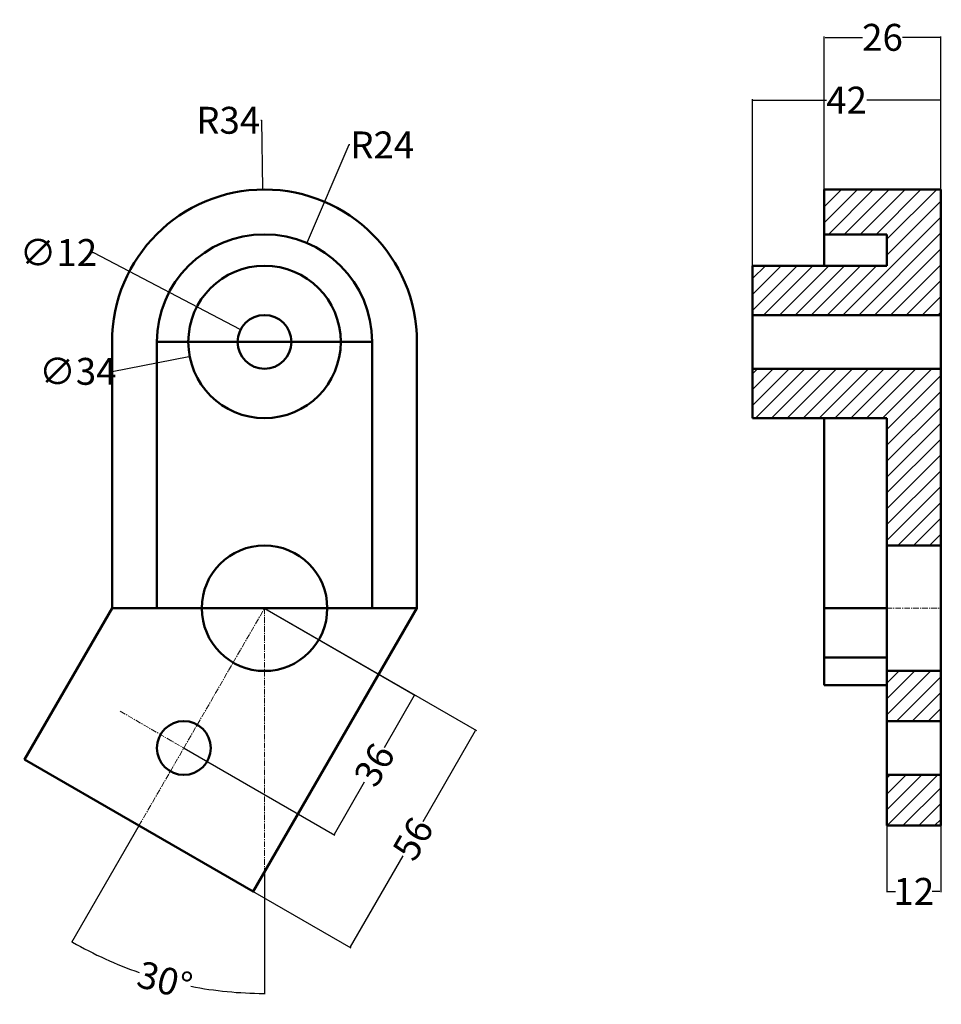
# Model space of a CAD drawing. Units: millimetres. Extents: x 37 to 242, y 56 to 275.
import ezdxf

# ---------------------------------------------------------------- set-up
doc = ezdxf.new("R2010")
doc.units = ezdxf.units.MM
doc.header["$MEASUREMENT"] = 0
doc.linetypes.add('CENTER', pattern=[2, 1.25, -0.25, 0.25, -0.25])
for name, color, linetype, lineweight in [('M-CNTR', 1, 'CENTER', 18), ('M-DIMS', 2, 'Continuous', 25), ('M-HATC', 8, 'Continuous', 18), ('M-OUTL', 7, 'Continuous', 50)]:
    doc.layers.add(name, color=color, linetype=linetype, lineweight=lineweight)
doc.styles.get("Standard").update_dxf_attribs({"font": 'arial.ttf'})
doc.dimstyles.get("Standard").update_dxf_attribs({"dimtxt": 6, "dimasz": 0.18, "dimexe": 0.18, "dimexo": 0.0625, "dimgap": 0.09, "dimtad": 0, "dimtoh": 1, "dimdec": 0, "dimzin": 0, "dimdsep": 46, "dimtxsty": 'Standard', "dimcen": 0.09, "dimadec": 0, "dimazin": 0, "dimtfac": 1, "dimtdec": 0, "dimtofl": 0, "dimtmove": 0, "dimatfit": 3, "dimfxl": 1, "dimtolj": 1, "dimtzin": 0, "dimarcsym": 0})

# ---------------------------------------------------------------- blocks, each defined once
blk = doc.blocks.new('*D1')
at = {"layer": 'Defpoints', "color": 0, "transparency": 16777216}
for p in [(90.71, 237.56), (91.17, 203.56)]:
    blk.add_point(p, dxfattribs=at)
at = {"layer": 'M-DIMS', "color": 0, "lineweight": -2, "transparency": 16777216}
for p, q in [((90.32, 253), (90.5, 253)), ((90.5, 253), (90.71, 237.74)), ((91.08, 203.56), (91.26, 203.56)), ((91.17, 203.47), (91.17, 203.65))]:
    blk.add_line(p, q, dxfattribs=at)
at = {"layer": 'M-DIMS', "color": 0, "transparency": 16777216}
blk.add_solid([(90.74, 237.74), (90.68, 237.74), (90.71, 237.56)], dxfattribs=at)
at = {"layer": 'M-DIMS', "color": 0, "transparency": 16777216, "insert": (83.07, 253), "char_height": 6, "attachment_point": 5}
blk.add_mtext('\\A1;R34', dxfattribs=at)
blk = doc.blocks.new('*D2')
at = {"layer": 'Defpoints', "color": 0, "transparency": 16777216}
for p in [(100.62, 225.62), (91.17, 203.56)]:
    blk.add_point(p, dxfattribs=at)
at = {"layer": 'M-DIMS', "color": 0, "lineweight": -2, "transparency": 16777216}
for p, q in [((110, 247.5), (100.69, 225.79)), ((110.18, 247.5), (110, 247.5)), ((91.08, 203.56), (91.26, 203.56)), ((91.17, 203.47), (91.17, 203.65))]:
    blk.add_line(p, q, dxfattribs=at)
at = {"layer": 'M-DIMS', "color": 0, "transparency": 16777216}
blk.add_solid([(100.67, 225.8), (100.72, 225.77), (100.62, 225.62)], dxfattribs=at)
at = {"layer": 'M-DIMS', "color": 0, "transparency": 16777216, "insert": (117.43, 247.5), "char_height": 6, "attachment_point": 5}
blk.add_mtext('\\A1;R24', dxfattribs=at)
blk = doc.blocks.new('*D3')
at = {"layer": 'Defpoints', "color": 0, "transparency": 16777216}
for p in [(242, 257.5), (200, 220.56), (242, 220.56)]:
    blk.add_point(p, dxfattribs=at)
at = {"layer": 'M-DIMS', "color": 0, "lineweight": -2, "transparency": 16777216}
for p, q in [((200, 220.62), (200, 257.68)), ((200.18, 257.5), (216.52, 257.5)), ((241.82, 257.5), (225.48, 257.5)), ((242, 220.62), (242, 257.68))]:
    blk.add_line(p, q, dxfattribs=at)
at = {"layer": 'M-DIMS', "color": 0, "transparency": 16777216}
for points in [[(200.18, 257.53), (200.18, 257.47), (200, 257.5)], [(241.82, 257.53), (241.82, 257.47), (242, 257.5)]]:
    blk.add_solid(points, dxfattribs=at)
at = {"layer": 'M-DIMS', "color": 0, "transparency": 16777216, "insert": (221, 257.5), "char_height": 6, "attachment_point": 5}
blk.add_mtext('\\A1;42', dxfattribs=at)
blk = doc.blocks.new('*D4')
at = {"layer": 'Defpoints', "color": 0, "transparency": 16777216}
for p in [(242, 271.5), (216, 237.56), (242, 237.56)]:
    blk.add_point(p, dxfattribs=at)
at = {"layer": 'M-DIMS', "color": 0, "lineweight": -2, "transparency": 16777216}
for p, q in [((216, 237.62), (216, 271.68)), ((216.18, 271.5), (224.56, 271.5)), ((241.82, 271.5), (233.44, 271.5)), ((242, 237.62), (242, 271.68))]:
    blk.add_line(p, q, dxfattribs=at)
at = {"layer": 'M-DIMS', "color": 0, "transparency": 16777216}
for points in [[(216.18, 271.53), (216.18, 271.47), (216, 271.5)], [(241.82, 271.53), (241.82, 271.47), (242, 271.5)]]:
    blk.add_solid(points, dxfattribs=at)
at = {"layer": 'M-DIMS', "color": 0, "transparency": 16777216, "insert": (229, 271.5), "char_height": 6, "attachment_point": 5}
blk.add_mtext('\\A1;26', dxfattribs=at)
blk = doc.blocks.new('*D5')
at = {"layer": 'Defpoints', "color": 0, "transparency": 16777216}
for p in [(230, 95.66), (242, 95.66), (242, 81)]:
    blk.add_point(p, dxfattribs=at)
at = {"layer": 'M-DIMS', "color": 0, "lineweight": -2, "transparency": 16777216}
for p, q in [((230, 95.6), (230, 80.82)), ((242, 95.6), (242, 80.82)), ((230.18, 81), (231.93, 81)), ((241.82, 81), (240.07, 81))]:
    blk.add_line(p, q, dxfattribs=at)
at = {"layer": 'M-DIMS', "color": 0, "transparency": 16777216}
for points in [[(230.18, 81.03), (230.18, 80.97), (230, 81)], [(241.82, 81.03), (241.82, 80.97), (242, 81)]]:
    blk.add_solid(points, dxfattribs=at)
at = {"layer": 'M-DIMS', "color": 0, "transparency": 16777216, "insert": (236, 81), "char_height": 6, "attachment_point": 5}
blk.add_mtext('\\A1;12', dxfattribs=at)
blk = doc.blocks.new('*D6')
at = {"layer": 'Defpoints', "color": 0, "transparency": 16777216}
for p in [(107.86, 206.78), (74.47, 200.34)]:
    blk.add_point(p, dxfattribs=at)
at = {"layer": 'M-DIMS', "color": 0, "lineweight": -2, "transparency": 16777216}
for p, q in [((91.08, 203.56), (91.26, 203.56)), ((91.17, 203.47), (91.17, 203.65)), ((57.17, 197), (74.3, 200.31))]:
    blk.add_line(p, q, dxfattribs=at)
at = {"layer": 'M-DIMS', "color": 0, "transparency": 16777216}
blk.add_solid([(74.29, 200.34), (74.3, 200.28), (74.47, 200.34)], dxfattribs=at)
at = {"layer": 'M-DIMS', "color": 0, "transparency": 16777216, "insert": (49.53, 197), "char_height": 6, "attachment_point": 5}
blk.add_mtext('\\A1;∅34', dxfattribs=at)
blk = doc.blocks.new('*D7')
at = {"layer": 'Defpoints', "color": 0, "transparency": 16777216}
for p in [(85.85, 206.34), (96.48, 200.78)]:
    blk.add_point(p, dxfattribs=at)
at = {"layer": 'M-DIMS', "color": 0, "lineweight": -2, "transparency": 16777216}
for p, q in [((52.82, 223.5), (53, 223.5)), ((53, 223.5), (85.69, 206.42)), ((91.08, 203.56), (91.26, 203.56)), ((91.17, 203.47), (91.17, 203.65))]:
    blk.add_line(p, q, dxfattribs=at)
at = {"layer": 'M-DIMS', "color": 0, "transparency": 16777216}
blk.add_solid([(85.7, 206.45), (85.68, 206.4), (85.85, 206.34)], dxfattribs=at)
at = {"layer": 'M-DIMS', "color": 0, "transparency": 16777216, "insert": (45.2, 223.5), "char_height": 6, "attachment_point": 5}
blk.add_mtext('\\A1;∅12', dxfattribs=at)
blk = doc.blocks.new('*D8')
at = {"layer": 'Defpoints', "color": 0, "transparency": 16777216}
for p in [(91.17, 144.16), (63.17, 95.66), (110.27, 68.47)]:
    blk.add_point(p, dxfattribs=at)
at = {"layer": 'M-DIMS', "color": 0, "lineweight": -2, "transparency": 16777216}
for p, q in [((91.22, 144.13), (138.42, 116.88)), ((138.18, 116.81), (126.46, 96.52)), ((63.22, 95.63), (110.42, 68.38)), ((110.36, 68.63), (122.07, 88.92))]:
    blk.add_line(p, q, dxfattribs=at)
at = {"layer": 'M-DIMS', "color": 0, "transparency": 16777216}
for points in [[(138.15, 116.83), (138.2, 116.8), (138.27, 116.97)], [(110.33, 68.64), (110.38, 68.61), (110.27, 68.47)]]:
    blk.add_solid(points, dxfattribs=at)
at = {"layer": 'M-DIMS', "color": 0, "transparency": 16777216, "insert": (124.27, 92.72), "char_height": 6, "attachment_point": 5, "rotation": 60}
blk.add_mtext('\\A1;56', dxfattribs=at)
blk = doc.blocks.new('*D9')
at = {"layer": 'Defpoints', "color": 0, "transparency": 16777216}
for p in [(91.17, 144.16), (73.17, 112.98), (106.66, 93.65)]:
    blk.add_point(p, dxfattribs=at)
at = {"layer": 'M-DIMS', "color": 0, "lineweight": -2, "transparency": 16777216}
for p, q in [((91.22, 144.13), (124.82, 124.73)), ((124.57, 124.67), (117.85, 113.03)), ((73.22, 112.95), (106.82, 93.56)), ((106.75, 93.8), (113.47, 105.44))]:
    blk.add_line(p, q, dxfattribs=at)
at = {"layer": 'M-DIMS', "color": 0, "transparency": 16777216}
for points in [[(124.55, 124.68), (124.6, 124.65), (124.66, 124.82)], [(106.73, 93.82), (106.78, 93.79), (106.66, 93.65)]]:
    blk.add_solid(points, dxfattribs=at)
at = {"layer": 'M-DIMS', "color": 0, "transparency": 16777216, "insert": (115.66, 109.23), "char_height": 6, "attachment_point": 5, "rotation": 60}
blk.add_mtext('\\A1;36', dxfattribs=at)
blk = doc.blocks.new('*D10')
at = {"layer": 'Defpoints', "color": 0, "transparency": 16777216}
for p in [(91.17, 144.16), (91.17, 144.16), (63.17, 95.66), (91.17, 85.27), (61.79, 63.44)]:
    blk.add_point(p, dxfattribs=at)
at = {"layer": 'M-DIMS', "color": 0, "lineweight": -2, "transparency": 16777216}
for p, q in [((63.14, 95.61), (48.12, 69.61)), ((91.17, 85.21), (91.17, 58.08))]:
    blk.add_line(p, q, dxfattribs=at)
for start, end in [(240.1201, 251.0128), (258.9872, 269.8799)]:
    blk.add_arc((91.17, 144.16), 85.91, start, end, dxfattribs=at)
at = {"layer": 'M-DIMS', "color": 0, "transparency": 16777216}
for points in [[(48.36, 69.65), (48.39, 69.7), (48.21, 69.77)], [(90.99, 58.29), (90.99, 58.23), (91.17, 58.26)]]:
    blk.add_solid(points, dxfattribs=at)
at = {"layer": 'M-DIMS', "color": 0, "transparency": 16777216, "insert": (68.93, 61.18), "char_height": 6, "attachment_point": 5, "rotation": 345}
blk.add_mtext('\\A1;30°', dxfattribs=at)

msp = doc.modelspace()

# ---------------------------------------------------------------- hatches: boundary and pattern name
at = {"layer": 'M-HATC'}
h = msp.add_hatch(dxfattribs=at)
h.set_pattern_fill('ANSI31', color=256, scale=20)
h.paths.add_polyline_path([(242, 237.56), (216, 237.56), (216, 227.56), (230, 227.56), (230, 220.56), (216, 220.56), (200, 220.56), (200, 209.56), (242, 209.56)])
h.paths.add_polyline_path([(242, 197.56), (200, 197.56), (200, 186.56), (230, 186.56), (230, 158.16), (242, 158.16), (242, 186.56)])
h.paths.add_polyline_path([(242, 130.16), (230, 130.16), (230, 118.98), (242, 118.98)])
h.paths.add_polyline_path([(242, 106.98), (230, 106.98), (230, 95.66), (242, 95.66)])

# ---------------------------------------------------------------- linework, layer by layer
at = {"layer": 'M-CNTR'}
for p, q in [((229.88, 144.16), (242.12, 144.16)), ((58.99, 121.17), (73.17, 112.98))]:
    msp.add_line(p, q, dxfattribs=at)
msp.add_lwpolyline([(63.17, 95.66), (91.17, 144.16), (91.17, 85.27)], dxfattribs=at)
at = {"layer": 'M-OUTL'}
for p, q in [((216, 237.56), (242, 237.56)), ((216, 237.56), (216, 220.56)), ((242, 237.56), (242, 186.56)), ((216, 227.56), (230, 227.56)), ((230, 227.56), (230, 220.56)), ((216, 220.56), (200, 220.56)), ((200, 220.56), (200, 186.56)), ((230, 220.56), (216, 220.56)), ((200, 209.56), (242, 209.56)), ((200, 197.56), (242, 197.56)), ((200, 186.56), (230, 186.56)), ((216, 186.56), (216, 127)), ((230, 186.56), (230, 158.16)), ((242, 158.16), (242, 186.56)), ((230, 158.16), (242, 158.16)), ((230, 158.16), (230, 118.98)), ((242, 130.16), (242, 158.16)), ((229.88, 144.16), (216, 144.16)), ((230, 133.16), (216, 133.16)), ((230, 131.16), (230, 131.16)), ((230, 130.16), (242, 130.16)), ((242, 130.16), (242, 118)), ((216, 127), (230, 127)), ((230, 118.98), (230, 95.66)), ((230, 118.98), (242, 118.98)), ((242, 118), (242, 95.66)), ((230, 106.98), (242, 106.98)), ((230, 95.66), (242, 95.66))]:
    msp.add_line(p, q, dxfattribs=at)
msp.add_lwpolyline([(57.17, 144.16), (57.17, 203.56, -1), (125.17, 203.56), (125.17, 144.16), (88.67, 80.94), (37.67, 110.39), (57.17, 144.16), (67.17, 144.16), (67.17, 203.56, -1), (115.17, 203.56)], format="xyb", dxfattribs=at)
for points in [[(67.17, 203.56), (115.17, 203.56), (115.17, 144.16)], [(67.17, 144.16), (115.17, 144.16), (125.17, 144.16)]]:
    msp.add_lwpolyline(points, dxfattribs=at)
for centre, radius in [((91.17, 203.56), 17), ((91.17, 203.56), 6), ((91.17, 144.16), 14), ((73.17, 112.98), 6)]:
    msp.add_circle(centre, radius, dxfattribs=at)

# ---------------------------------------------------------------- dimensions: what is measured, and where the dimension line sits
at = {"layer": 'M-DIMS'}
for base, p1, p2, picture, middle in [((242, 271.5), (216, 237.56), (242, 237.56), '*D4', (229, 271.5)), ((242, 257.5), (200, 220.56), (242, 220.56), '*D3', (221, 257.5)), ((242, 81), (230, 95.66), (242, 95.66), '*D5', (236, 81))]:
    dim = msp.add_linear_dim(base=base, p1=p1, p2=p2, dimstyle='Standard', override={"dimclrd": 0, "dimclre": 0, "dimclrt": 0}, dxfattribs=at)
    dim.commit()
    dim.dimension.update_dxf_attribs({"geometry": picture, "text_midpoint": middle})
for mpoint, picture, middle in [((90.71, 237.56), '*D1', (83.07, 253)), ((100.62, 225.62), '*D2', (117.43, 247.5))]:
    dim = msp.add_radius_dim(center=(91.17, 203.56), mpoint=mpoint, dimstyle='Standard', override={"dimclrd": 0, "dimclre": 0, "dimclrt": 0}, dxfattribs=at)
    dim.commit()
    dim.dimension.update_dxf_attribs({"geometry": picture, "text_midpoint": middle, "dimtype": 164})
for p1, p2, picture, middle in [((96.48, 200.78), (85.85, 206.34), '*D7', (45.2, 223.5)), ((107.86, 206.78), (74.47, 200.34), '*D6', (57.17, 197))]:
    dim = msp.add_diameter_dim_2p(p1=p1, p2=p2, dimstyle='Standard', override={"dimclrd": 0, "dimclre": 0, "dimclrt": 0}, dxfattribs=at)
    dim.commit()
    dim.dimension.update_dxf_attribs({"geometry": picture, "text_midpoint": middle, "dimtype": 163})
dim = msp.add_angular_dim_2l(base=(61.79, 63.44), line1=((63.17, 95.66), (91.17, 144.16)), line2=((91.17, 144.16), (91.17, 85.27)), dimstyle='Standard', override={"dimclrd": 0, "dimclre": 0, "dimclrt": 0}, dxfattribs=at)
dim.commit()
dim.dimension.update_dxf_attribs({"geometry": '*D10', "text_midpoint": (68.93, 61.18)})
for p2, distance, picture, middle in [((63.17, 95.66), 54.39, '*D8', (124.27, 92.72)), ((73.17, 112.98), 38.68, '*D9', (115.66, 109.23))]:
    dim = msp.add_aligned_dim(p1=(91.17, 144.16), p2=p2, distance=distance, dimstyle='Standard', override={"dimclrd": 0, "dimclre": 0, "dimclrt": 0}, dxfattribs=at)
    dim.commit()
    dim.dimension.update_dxf_attribs({"geometry": picture, "text_midpoint": middle})

doc.saveas('drawing.dxf')
